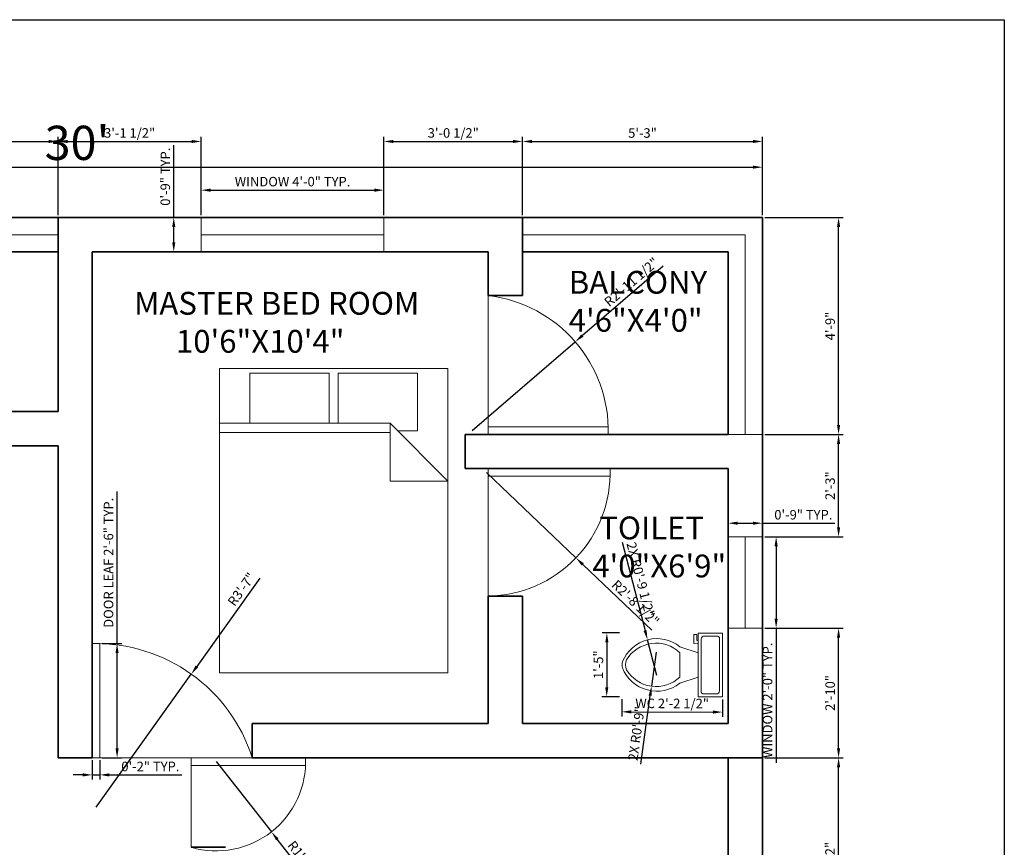
# Model space of a CAD drawing. Units: inches. Extents: x 5717 to 6221, y 11359 to 11763.
# Tile 4 of 4: x 5963 to 6221, y 11546 to 11763. Entities that reach past the tile are written whole.
import ezdxf

# ---------------------------------------------------------------- set-up
doc = ezdxf.new("R2010")
doc.units = ezdxf.units.IN
for name, color, linetype, lineweight, true_color in [('A-ANNO-DIMS', 254, 'Continuous', 13, 0xfeeab9), ('A-ANNO-TTLB', 51, 'Continuous', 25, 0xf8f6b0), ('A-AREA-IDEN', 11, 'Continuous', 20, 0xf27172), ('A-WALL', 244, 'Continuous', 35, 0x991b1e)]:
    doc.layers.add(name, color=color, linetype=linetype, lineweight=lineweight, true_color=true_color)
for name, color, linetype, lineweight in [('A-DOOR', 5, 'Continuous', 18), ('A-FLOR-FIXT', 1, 'Continuous', 18), ('A-FURN', 8, 'Continuous', 18), ('A-GLAZ', 4, 'Continuous', 18)]:
    doc.layers.add(name, color=color, linetype=linetype, lineweight=lineweight)
doc.styles.get("Standard").update_dxf_attribs({"font": 'arial.ttf'})
doc.dimstyles.new('ISO-25', dxfattribs={"dimtxt": 2.5, "dimasz": 2.5, "dimexe": 1.25, "dimexo": 0.625, "dimtad": 1, "dimlunit": 3, "dimtxsty": 'Standard', "dimcen": 2.5, "dimadec": 0, "dimazin": 0, "dimtfac": 1, "dimtmove": 0, "dimatfit": 3, "dimfxl": 1, "dimarcsym": 0})

# ---------------------------------------------------------------- blocks, each defined once
blk = doc.blocks.new('*D12')
at = {"layer": 'A-ANNO-DIMS', "color": 0, "lineweight": -2, "transparency": 16777216}
for p, q in [((5797.9, 11711.73), (5797.9, 11725.6)), ((6157.9, 11711.73), (6157.9, 11725.6)), ((5800.4, 11724.35), (6155.4, 11724.35))]:
    blk.add_line(p, q, dxfattribs=at)
at = {"layer": 'A-ANNO-DIMS', "color": 0, "transparency": 16777216}
for points in [[(5800.4, 11724.77), (5800.4, 11723.94), (5797.9, 11724.35)], [(6155.4, 11724.77), (6155.4, 11723.94), (6157.9, 11724.35)]]:
    blk.add_solid(points, dxfattribs=at)
at = {"layer": 'Defpoints', "color": 0, "transparency": 16777216}
for p in [(6157.9, 11724.35), (5797.9, 11711.11), (6157.9, 11711.11)]:
    blk.add_point(p, dxfattribs=at)
at = {"layer": 'A-ANNO-DIMS', "color": 0, "transparency": 16777216, "insert": (5977.9, 11729.58), "char_height": 9, "attachment_point": 5}
blk.add_mtext("30'", dxfattribs=at)
blk = doc.blocks.new('Toilet - top')
for p, q in [((9.5, -6), (9.5, -2)), ((-10, -8.5), (-8, -8.5)), ((-10, -9.5), (-10, -8.5)), ((-7, -9.5), (-10, -9.5)), ((-8, -8.5), (-8, -8)), ((-7, -8), (-7, -9.5)), ((-4, -8), (-6, -14)), ((4, -8), (6, -14)), ((4, -14), (-4, -14))]:
    blk.add_line(p, q)
blk.add_lwpolyline([(10.5, -8), (10.5, 0), (-10.5, 0), (-10.5, -8)], close=True)
for points in [[(-9.5, -2), (-9.5, -6)], [(8.5, -1), (-8.5, -1)], [(-8.5, -7), (8.5, -7)]]:
    blk.add_lwpolyline(points)
for centre, radius, start, end in [((-8.62, -1.88), 0.884, 81.8699, 188.1301), ((8.62, -1.88), 0.884, 351.8699, 98.1301), ((-8.62, -6.12), 0.884, 171.8699, 278.1301), ((8.62, -6.12), 0.884, 261.8699, 8.1301), ((3.52, -21.58), 12.17, 141.4691, 247.9714), ((4.2, -21.82), 11.33, 136.3677, 238.9468), ((-3.52, -21.58), 12.17, 292.0284, 38.5307), ((-4.2, -21.82), 11.33, 301.053, 43.6321), ((0, -27.88), 4, 245.7318, 294.2682), ((0, -29), 4, 254.8605, 285.1395)]:
    blk.add_arc(centre, radius, start, end)
blk = doc.blocks.new('Bed - Queen')
for p, q in [((0, -80.00003), (0, 0)), ((0, 0), (59.99999, 0)), ((59.99999, 0), (59.99999, -80.00003)), ((7.99999, -1.2), (28.79998, -1.2)), ((7.99999, -14.4), (7.99999, -1.2)), ((28.79998, -1.2), (28.79998, -14.4)), ((31.19999, -1.2), (51.99999, -1.2)), ((31.19999, -14.4), (31.19999, -1.2)), ((51.99999, -1.2), (51.99999, -16.4)), ((0, -14.4), (44.8, -14.4)), ((59.99999, -29.6), (44.8, -14.4)), ((44.8, -14.4), (44.8, -29.6)), ((44.8, -16.8), (0, -16.8)), ((51.99999, -16.4), (46.79936, -16.4)), ((44.8, -29.6), (59.99999, -29.6)), ((59.99999, -80.00003), (0, -80.00003))]:
    blk.add_line(p, q)
blk = doc.blocks.new('DOOR-LEAF-30IN')
for p, q in [((2, 30), (0, 30)), ((0, 30), (0, 0)), ((2, 0), (2, 30))]:
    blk.add_line(p, q)
blk = doc.blocks.new('WIN-24IN')
for p, q in [((0, 9), (0, 0)), ((24, 9), (0, 9)), ((24, 9), (24, 0)), ((24, 0), (24, 9)), ((0, 4.5), (24, 4.5)), ((0, 0), (24, 0))]:
    blk.add_line(p, q)
blk = doc.blocks.new('WIN-48IN')
for p, q in [((0, 0), (0, 9)), ((0, 9), (48, 9)), ((48, 9), (48, 0)), ((0, 4.5), (48, 4.5)), ((48, 0), (0, 0))]:
    blk.add_line(p, q)
blk = doc.blocks.new('*D18')
at = {"layer": 'A-ANNO-DIMS', "color": 0, "lineweight": -2, "transparency": 16777216}
for p, q in [((5988.4, 11599.11), (5988.4, 11639.13)), ((5984.53, 11599.11), (5989.65, 11599.11)), ((5988.4, 11571.61), (5988.4, 11596.61)), ((5984.53, 11569.11), (5989.65, 11569.11))]:
    blk.add_line(p, q, dxfattribs=at)
at = {"layer": 'A-ANNO-DIMS', "color": 0, "transparency": 16777216}
for points in [[(5987.99, 11596.61), (5988.82, 11596.61), (5988.4, 11599.11)], [(5987.99, 11571.61), (5988.82, 11571.61), (5988.4, 11569.11)]]:
    blk.add_solid(points, dxfattribs=at)
at = {"layer": 'Defpoints', "color": 0, "transparency": 16777216}
for p in [(5983.9, 11599.11), (5988.4, 11599.11), (5983.9, 11569.11)]:
    blk.add_point(p, dxfattribs=at)
at = {"layer": 'A-ANNO-DIMS', "color": 0, "transparency": 16777216, "insert": (5986.48, 11620.37), "char_height": 2.5, "attachment_point": 5, "rotation": 90}
blk.add_mtext('DOOR LEAF 2\'-6" TYP.', dxfattribs=at)
blk = doc.blocks.new('*D19')
at = {"layer": 'A-ANNO-DIMS', "color": 0, "lineweight": -2, "transparency": 16777216}
for p, q in [((5981.9, 11568.48), (5981.9, 11563.36)), ((5983.9, 11568.48), (5983.9, 11563.36)), ((5979.4, 11564.61), (5976.9, 11564.61)), ((5981.9, 11564.61), (5983.9, 11564.61)), ((5986.4, 11564.61), (6005.39, 11564.61))]:
    blk.add_line(p, q, dxfattribs=at)
at = {"layer": 'A-ANNO-DIMS', "color": 0, "transparency": 16777216}
for points in [[(5979.4, 11565.03), (5979.4, 11564.19), (5981.9, 11564.61)], [(5986.4, 11565.03), (5986.4, 11564.19), (5983.9, 11564.61)]]:
    blk.add_solid(points, dxfattribs=at)
at = {"layer": 'Defpoints', "color": 0, "transparency": 16777216}
for p in [(5981.9, 11569.11), (5983.9, 11569.11), (5983.9, 11564.61)]:
    blk.add_point(p, dxfattribs=at)
at = {"layer": 'A-ANNO-DIMS', "color": 0, "transparency": 16777216, "insert": (5997.15, 11566.51), "char_height": 2.5, "attachment_point": 5}
blk.add_mtext('0\'-2" TYP.', dxfattribs=at)
blk = doc.blocks.new('*D24')
at = {"layer": 'A-ANNO-DIMS', "color": 0, "lineweight": -2, "transparency": 16777216}
for p, q in [((6158.53, 11627.17), (6162.75, 11627.17)), ((6161.5, 11624.67), (6161.5, 11605.67)), ((6158.53, 11603.17), (6162.75, 11603.17)), ((6161.5, 11603.17), (6161.5, 11567.78))]:
    blk.add_line(p, q, dxfattribs=at)
at = {"layer": 'A-ANNO-DIMS', "color": 0, "transparency": 16777216}
for points in [[(6161.09, 11624.67), (6161.92, 11624.67), (6161.5, 11627.17)], [(6161.09, 11605.67), (6161.92, 11605.67), (6161.5, 11603.17)]]:
    blk.add_solid(points, dxfattribs=at)
at = {"layer": 'Defpoints', "color": 0, "transparency": 16777216}
for p in [(6157.9, 11627.17), (6157.9, 11603.17), (6161.5, 11603.17)]:
    blk.add_point(p, dxfattribs=at)
at = {"layer": 'A-ANNO-DIMS', "color": 0, "transparency": 16777216, "insert": (6159.58, 11584.22), "char_height": 2.5, "attachment_point": 5, "rotation": 90}
blk.add_mtext('WINDOW 2\'-0" TYP.', dxfattribs=at)
blk = doc.blocks.new('*D25')
at = {"layer": 'A-ANNO-DIMS', "color": 0, "lineweight": -2, "transparency": 16777216}
for p, q in [((6148.9, 11627.79), (6148.9, 11632.02)), ((6151.4, 11630.77), (6155.4, 11630.77)), ((6157.9, 11627.79), (6157.9, 11632.02)), ((6157.9, 11630.77), (6176.89, 11630.77))]:
    blk.add_line(p, q, dxfattribs=at)
at = {"layer": 'A-ANNO-DIMS', "color": 0, "transparency": 16777216}
for points in [[(6151.4, 11631.18), (6151.4, 11630.35), (6148.9, 11630.77)], [(6155.4, 11631.18), (6155.4, 11630.35), (6157.9, 11630.77)]]:
    blk.add_solid(points, dxfattribs=at)
at = {"layer": 'Defpoints', "color": 0, "transparency": 16777216}
for p in [(6157.9, 11630.77), (6148.9, 11627.17), (6157.9, 11627.17)]:
    blk.add_point(p, dxfattribs=at)
at = {"layer": 'A-ANNO-DIMS', "color": 0, "transparency": 16777216, "insert": (6168.65, 11632.67), "char_height": 2.5, "attachment_point": 5}
blk.add_mtext('0\'-9" TYP.', dxfattribs=at)
blk = doc.blocks.new('*D26')
at = {"layer": 'A-ANNO-DIMS', "color": 0, "lineweight": -2, "transparency": 16777216}
for p, q in [((6010.49, 11711.73), (6010.49, 11719.56)), ((6012.99, 11718.31), (6055.99, 11718.31)), ((6058.49, 11711.73), (6058.49, 11719.56))]:
    blk.add_line(p, q, dxfattribs=at)
at = {"layer": 'A-ANNO-DIMS', "color": 0, "transparency": 16777216}
for points in [[(6012.99, 11718.73), (6012.99, 11717.89), (6010.49, 11718.31)], [(6055.99, 11718.73), (6055.99, 11717.89), (6058.49, 11718.31)]]:
    blk.add_solid(points, dxfattribs=at)
at = {"layer": 'Defpoints', "color": 0, "transparency": 16777216}
for p in [(6058.49, 11718.31), (6010.49, 11711.11), (6058.49, 11711.11)]:
    blk.add_point(p, dxfattribs=at)
at = {"layer": 'A-ANNO-DIMS', "color": 0, "transparency": 16777216, "insert": (6034.49, 11720.23), "char_height": 2.5, "attachment_point": 5}
blk.add_mtext('WINDOW 4\'-0" TYP.', dxfattribs=at)
blk = doc.blocks.new('*D27')
at = {"layer": 'A-ANNO-DIMS', "color": 0, "lineweight": -2, "transparency": 16777216}
for p, q in [((6003.29, 11711.11), (6003.29, 11730.1)), ((6009.87, 11711.11), (6002.04, 11711.11)), ((6003.29, 11704.61), (6003.29, 11708.61)), ((6009.87, 11702.11), (6002.04, 11702.11))]:
    blk.add_line(p, q, dxfattribs=at)
at = {"layer": 'A-ANNO-DIMS', "color": 0, "transparency": 16777216}
for points in [[(6002.87, 11708.61), (6003.71, 11708.61), (6003.29, 11711.11)], [(6002.87, 11704.61), (6003.71, 11704.61), (6003.29, 11702.11)]]:
    blk.add_solid(points, dxfattribs=at)
at = {"layer": 'Defpoints', "color": 0, "transparency": 16777216}
for p in [(6003.29, 11711.11), (6010.49, 11711.11), (6010.49, 11702.11)]:
    blk.add_point(p, dxfattribs=at)
at = {"layer": 'A-ANNO-DIMS', "color": 0, "transparency": 16777216, "insert": (6001.39, 11721.85), "char_height": 2.5, "attachment_point": 5, "rotation": 90}
blk.add_mtext('0\'-9" TYP.', dxfattribs=at)
blk = doc.blocks.new('*D30')
at = {"layer": 'A-ANNO-DIMS', "color": 0, "lineweight": -2, "transparency": 16777216}
for p, q in [((6120.97, 11584.53), (6120.96, 11579.94)), ((6147.41, 11584.46), (6147.4, 11579.87)), ((6123.46, 11581.18), (6144.9, 11581.13))]:
    blk.add_line(p, q, dxfattribs=at)
at = {"layer": 'A-ANNO-DIMS', "color": 0, "transparency": 16777216}
for points in [[(6123.46, 11581.6), (6123.46, 11580.77), (6120.96, 11581.19)], [(6144.9, 11581.55), (6144.9, 11580.71), (6147.4, 11581.12)]]:
    blk.add_solid(points, dxfattribs=at)
at = {"layer": 'Defpoints', "color": 0, "transparency": 16777216}
for p in [(6120.97, 11585.15), (6147.41, 11585.09), (6147.4, 11581.12)]:
    blk.add_point(p, dxfattribs=at)
at = {"layer": 'A-ANNO-DIMS', "color": 0, "transparency": 16777216, "insert": (6134.19, 11583.07), "char_height": 2.5, "attachment_point": 5, "rotation": 359.8573}
blk.add_mtext('WC 2\'-2 1/2"', dxfattribs=at)
blk = doc.blocks.new('*D31')
at = {"layer": 'A-ANNO-DIMS', "color": 0, "lineweight": -2, "transparency": 16777216}
for p, q in [((6120.39, 11601.96), (6115.8, 11601.97)), ((6117.04, 11599.46), (6117.01, 11587.66)), ((6120.35, 11585.16), (6115.76, 11585.17))]:
    blk.add_line(p, q, dxfattribs=at)
at = {"layer": 'A-ANNO-DIMS', "color": 0, "transparency": 16777216}
for points in [[(6116.63, 11599.47), (6117.46, 11599.46), (6117.05, 11601.96)], [(6116.6, 11587.67), (6117.43, 11587.66), (6117.01, 11585.16)]]:
    blk.add_solid(points, dxfattribs=at)
at = {"layer": 'Defpoints', "color": 0, "transparency": 16777216}
for p in [(6121.02, 11601.95), (6117.01, 11585.16), (6120.97, 11585.15)]:
    blk.add_point(p, dxfattribs=at)
at = {"layer": 'A-ANNO-DIMS', "color": 0, "transparency": 16777216, "insert": (6115.13, 11593.57), "char_height": 2.5, "attachment_point": 5, "rotation": 89.8573}
blk.add_mtext('1\'-5"', dxfattribs=at)
blk = doc.blocks.new('*D43')
at = {"layer": 'A-ANNO-DIMS', "color": 0, "lineweight": -2, "transparency": 16777216}
for p, q in [((6158.53, 11569.11), (6179.15, 11569.11)), ((6177.9, 11513.97), (6177.9, 11566.61)), ((6158.53, 11511.47), (6179.15, 11511.47))]:
    blk.add_line(p, q, dxfattribs=at)
at = {"layer": 'A-ANNO-DIMS', "color": 0, "transparency": 16777216}
for points in [[(6177.49, 11566.61), (6178.32, 11566.61), (6177.9, 11569.11)], [(6177.49, 11513.97), (6178.32, 11513.97), (6177.9, 11511.47)]]:
    blk.add_solid(points, dxfattribs=at)
at = {"layer": 'Defpoints', "color": 0, "transparency": 16777216}
for p in [(6157.9, 11569.11), (6177.9, 11569.11), (6157.9, 11511.47)]:
    blk.add_point(p, dxfattribs=at)
at = {"layer": 'A-ANNO-DIMS', "color": 0, "transparency": 16777216, "insert": (6175.98, 11540.29), "char_height": 2.5, "attachment_point": 5, "rotation": 90}
blk.add_mtext('4\'-9 1/2"', dxfattribs=at)
blk = doc.blocks.new('*D44')
at = {"layer": 'A-ANNO-DIMS', "color": 0, "lineweight": -2, "transparency": 16777216}
for p, q in [((6158.53, 11603.17), (6179.15, 11603.17)), ((6177.9, 11571.61), (6177.9, 11600.67)), ((6158.53, 11569.11), (6179.15, 11569.11))]:
    blk.add_line(p, q, dxfattribs=at)
at = {"layer": 'A-ANNO-DIMS', "color": 0, "transparency": 16777216}
for points in [[(6177.49, 11600.67), (6178.32, 11600.67), (6177.9, 11603.17)], [(6177.49, 11571.61), (6178.32, 11571.61), (6177.9, 11569.11)]]:
    blk.add_solid(points, dxfattribs=at)
at = {"layer": 'Defpoints', "color": 0, "transparency": 16777216}
for p in [(6157.9, 11603.17), (6177.9, 11603.17), (6157.9, 11569.11)]:
    blk.add_point(p, dxfattribs=at)
at = {"layer": 'A-ANNO-DIMS', "color": 0, "transparency": 16777216, "insert": (6176, 11586.14), "char_height": 2.5, "attachment_point": 5, "rotation": 90}
blk.add_mtext('2\'-10"', dxfattribs=at)
blk = doc.blocks.new('*D45')
at = {"layer": 'A-ANNO-DIMS', "color": 0, "lineweight": -2, "transparency": 16777216}
for p, q in [((6158.53, 11654.11), (6179.15, 11654.11)), ((6177.9, 11629.67), (6177.9, 11651.61)), ((6158.53, 11627.17), (6179.15, 11627.17))]:
    blk.add_line(p, q, dxfattribs=at)
at = {"layer": 'A-ANNO-DIMS', "color": 0, "transparency": 16777216}
for points in [[(6177.49, 11651.61), (6178.32, 11651.61), (6177.9, 11654.11)], [(6177.49, 11629.67), (6178.32, 11629.67), (6177.9, 11627.17)]]:
    blk.add_solid(points, dxfattribs=at)
at = {"layer": 'Defpoints', "color": 0, "transparency": 16777216}
for p in [(6157.9, 11654.11), (6177.9, 11654.11), (6157.9, 11627.17)]:
    blk.add_point(p, dxfattribs=at)
at = {"layer": 'A-ANNO-DIMS', "color": 0, "transparency": 16777216, "insert": (6176, 11640.64), "char_height": 2.5, "attachment_point": 5, "rotation": 90}
blk.add_mtext('2\'-3"', dxfattribs=at)
blk = doc.blocks.new('*D46')
at = {"layer": 'A-ANNO-DIMS', "color": 0, "lineweight": -2, "transparency": 16777216}
for p, q in [((6158.53, 11711.11), (6179.15, 11711.11)), ((6177.9, 11656.61), (6177.9, 11708.61)), ((6158.53, 11654.11), (6179.15, 11654.11))]:
    blk.add_line(p, q, dxfattribs=at)
at = {"layer": 'A-ANNO-DIMS', "color": 0, "transparency": 16777216}
for points in [[(6177.49, 11708.61), (6178.32, 11708.61), (6177.9, 11711.11)], [(6177.49, 11656.61), (6178.32, 11656.61), (6177.9, 11654.11)]]:
    blk.add_solid(points, dxfattribs=at)
at = {"layer": 'Defpoints', "color": 0, "transparency": 16777216}
for p in [(6157.9, 11711.11), (6177.9, 11711.11), (6157.9, 11654.11)]:
    blk.add_point(p, dxfattribs=at)
at = {"layer": 'A-ANNO-DIMS', "color": 0, "transparency": 16777216, "insert": (6176, 11682.61), "char_height": 2.5, "attachment_point": 5, "rotation": 90}
blk.add_mtext('4\'-9"', dxfattribs=at)
blk = doc.blocks.new('*D51')
at = {"layer": 'A-ANNO-DIMS', "color": 0, "lineweight": -2, "transparency": 16777216}
for p, q in [((5886.11, 11711.73), (5886.11, 11732.36)), ((5888.61, 11731.11), (5970.4, 11731.11)), ((5972.9, 11711.73), (5972.9, 11732.36))]:
    blk.add_line(p, q, dxfattribs=at)
at = {"layer": 'A-ANNO-DIMS', "color": 0, "transparency": 16777216}
for points in [[(5888.61, 11731.53), (5888.61, 11730.69), (5886.11, 11731.11)], [(5970.4, 11731.53), (5970.4, 11730.69), (5972.9, 11731.11)]]:
    blk.add_solid(points, dxfattribs=at)
at = {"layer": 'Defpoints', "color": 0, "transparency": 16777216}
for p in [(5972.9, 11731.11), (5886.11, 11711.11), (5972.9, 11711.11)]:
    blk.add_point(p, dxfattribs=at)
at = {"layer": 'A-ANNO-DIMS', "color": 0, "transparency": 16777216, "insert": (5929.51, 11733.01), "char_height": 2.5, "attachment_point": 5}
blk.add_mtext('7\'-3"', dxfattribs=at)
blk = doc.blocks.new('*D52')
at = {"layer": 'A-ANNO-DIMS', "color": 0, "lineweight": -2, "transparency": 16777216}
for p, q in [((5972.9, 11711.73), (5972.9, 11732.36)), ((5975.4, 11731.11), (6007.99, 11731.11)), ((6010.49, 11711.73), (6010.49, 11732.36))]:
    blk.add_line(p, q, dxfattribs=at)
at = {"layer": 'A-ANNO-DIMS', "color": 0, "transparency": 16777216}
for points in [[(5975.4, 11731.53), (5975.4, 11730.69), (5972.9, 11731.11)], [(6007.99, 11731.53), (6007.99, 11730.69), (6010.49, 11731.11)]]:
    blk.add_solid(points, dxfattribs=at)
at = {"layer": 'Defpoints', "color": 0, "transparency": 16777216}
for p in [(6010.49, 11731.11), (5972.9, 11711.11), (6010.49, 11711.11)]:
    blk.add_point(p, dxfattribs=at)
at = {"layer": 'A-ANNO-DIMS', "color": 0, "transparency": 16777216, "insert": (5991.7, 11733.03), "char_height": 2.5, "attachment_point": 5}
blk.add_mtext('3\'-1 1/2"', dxfattribs=at)
blk = doc.blocks.new('*D53')
at = {"layer": 'A-ANNO-DIMS', "color": 0, "lineweight": -2, "transparency": 16777216}
for p, q in [((6058.49, 11711.73), (6058.49, 11732.36)), ((6060.99, 11731.11), (6092.4, 11731.11)), ((6094.9, 11711.73), (6094.9, 11732.36))]:
    blk.add_line(p, q, dxfattribs=at)
at = {"layer": 'A-ANNO-DIMS', "color": 0, "transparency": 16777216}
for points in [[(6060.99, 11731.53), (6060.99, 11730.69), (6058.49, 11731.11)], [(6092.4, 11731.53), (6092.4, 11730.69), (6094.9, 11731.11)]]:
    blk.add_solid(points, dxfattribs=at)
at = {"layer": 'Defpoints', "color": 0, "transparency": 16777216}
for p in [(6094.9, 11731.11), (6058.49, 11711.11), (6094.9, 11711.11)]:
    blk.add_point(p, dxfattribs=at)
at = {"layer": 'A-ANNO-DIMS', "color": 0, "transparency": 16777216, "insert": (6076.7, 11733.03), "char_height": 2.5, "attachment_point": 5}
blk.add_mtext('3\'-0 1/2"', dxfattribs=at)
blk = doc.blocks.new('*D54')
at = {"layer": 'A-ANNO-DIMS', "color": 0, "lineweight": -2, "transparency": 16777216}
for p, q in [((6094.9, 11711.73), (6094.9, 11732.36)), ((6097.4, 11731.11), (6155.4, 11731.11)), ((6157.9, 11711.73), (6157.9, 11732.36))]:
    blk.add_line(p, q, dxfattribs=at)
at = {"layer": 'A-ANNO-DIMS', "color": 0, "transparency": 16777216}
for points in [[(6097.4, 11731.53), (6097.4, 11730.69), (6094.9, 11731.11)], [(6155.4, 11731.53), (6155.4, 11730.69), (6157.9, 11731.11)]]:
    blk.add_solid(points, dxfattribs=at)
at = {"layer": 'Defpoints', "color": 0, "transparency": 16777216}
for p in [(6157.9, 11731.11), (6094.9, 11711.11), (6157.9, 11711.11)]:
    blk.add_point(p, dxfattribs=at)
at = {"layer": 'A-ANNO-DIMS', "color": 0, "transparency": 16777216, "insert": (6126.4, 11733.01), "char_height": 2.5, "attachment_point": 5}
blk.add_mtext('5\'-3"', dxfattribs=at)
blk = doc.blocks.new('*D60')
at = {"layer": 'A-ANNO-DIMS', "color": 0, "lineweight": -2, "transparency": 16777216}
for p, q in [((6025.89, 11616.3), (6009.36, 11593.14)), ((5982.9, 11556.11), (6007.9, 11591.11))]:
    blk.add_line(p, q, dxfattribs=at)
at = {"layer": 'A-ANNO-DIMS', "color": 0, "transparency": 16777216}
blk.add_solid([(6009.02, 11593.39), (6009.69, 11592.9), (6007.9, 11591.11)], dxfattribs=at)
at = {"layer": 'Defpoints', "color": 0, "transparency": 16777216}
for p in [(6007.9, 11591.11), (5982.9, 11556.11)]:
    blk.add_point(p, dxfattribs=at)
at = {"layer": 'A-ANNO-DIMS', "color": 0, "transparency": 16777216, "insert": (6021.35, 11613.21), "char_height": 2.5, "attachment_point": 5, "rotation": 54.4628}
blk.add_mtext('R3\'-7"', dxfattribs=at)
blk = doc.blocks.new('*D61')
at = {"layer": 'A-ANNO-DIMS', "color": 0, "lineweight": -2, "transparency": 16777216}
for p, q in [((6131.79, 11698.37), (6110.62, 11680.09)), ((6081.69, 11655.11), (6108.73, 11678.46))]:
    blk.add_line(p, q, dxfattribs=at)
at = {"layer": 'A-ANNO-DIMS', "color": 0, "transparency": 16777216}
blk.add_solid([(6110.35, 11680.41), (6110.89, 11679.78), (6108.73, 11678.46)], dxfattribs=at)
at = {"layer": 'Defpoints', "color": 0, "transparency": 16777216}
for p in [(6108.73, 11678.46), (6081.69, 11655.11)]:
    blk.add_point(p, dxfattribs=at)
at = {"layer": 'A-ANNO-DIMS', "color": 0, "transparency": 16777216, "insert": (6123.7, 11693.92), "char_height": 2.5, "attachment_point": 5, "rotation": 40.8133}
blk.add_mtext('R2\'-11 1/2"', dxfattribs=at)
blk = doc.blocks.new('*D62')
at = {"layer": 'A-ANNO-DIMS', "color": 0, "lineweight": -2, "transparency": 16777216}
for p, q in [((6085.41, 11644.11), (6108.92, 11621.66)), ((6128.85, 11602.62), (6110.73, 11619.93))]:
    blk.add_line(p, q, dxfattribs=at)
at = {"layer": 'A-ANNO-DIMS', "color": 0, "transparency": 16777216}
blk.add_solid([(6111.01, 11620.23), (6110.44, 11619.63), (6108.92, 11621.66)], dxfattribs=at)
at = {"layer": 'Defpoints', "color": 0, "transparency": 16777216}
for p in [(6085.41, 11644.11), (6108.92, 11621.66)]:
    blk.add_point(p, dxfattribs=at)
at = {"layer": 'A-ANNO-DIMS', "color": 0, "transparency": 16777216, "insert": (6124.35, 11609.57), "char_height": 2.5, "attachment_point": 5, "rotation": 316.3127}
blk.add_mtext('R2\'-8 1/2"', dxfattribs=at)
blk = doc.blocks.new('*D66')
at = {"layer": 'A-ANNO-DIMS', "color": 0, "lineweight": -2, "transparency": 16777216}
for p, q in [((6014.46, 11568.11), (6028.94, 11549.64)), ((6043.2, 11531.46), (6030.48, 11547.68))]:
    blk.add_line(p, q, dxfattribs=at)
at = {"layer": 'A-ANNO-DIMS', "color": 0, "transparency": 16777216}
blk.add_solid([(6030.81, 11547.93), (6030.16, 11547.42), (6028.94, 11549.64)], dxfattribs=at)
at = {"layer": 'Defpoints', "color": 0, "transparency": 16777216}
for p in [(6014.46, 11568.11), (6028.94, 11549.64)]:
    blk.add_point(p, dxfattribs=at)
at = {"layer": 'A-ANNO-DIMS', "color": 0, "transparency": 16777216, "insert": (6039.14, 11539.75), "char_height": 2.5, "attachment_point": 5, "rotation": 308.1145}
blk.add_mtext('R1\'-11 1/2"', dxfattribs=at)
blk = doc.blocks.new('*D70')
at = {"layer": 'A-ANNO-DIMS', "color": 0, "lineweight": -2, "transparency": 16777216}
for p, q in [((6121.03, 11625.81), (6127.08, 11602.56)), ((6130.16, 11590.72), (6127.71, 11600.14))]:
    blk.add_line(p, q, dxfattribs=at)
at = {"layer": 'A-ANNO-DIMS', "color": 0, "transparency": 16777216}
blk.add_solid([(6127.48, 11602.66), (6126.68, 11602.45), (6127.71, 11600.14)], dxfattribs=at)
at = {"layer": 'Defpoints', "color": 0, "transparency": 16777216}
for p in [(6127.71, 11600.14), (6130.16, 11590.72)]:
    blk.add_point(p, dxfattribs=at)
at = {"layer": 'A-ANNO-DIMS', "color": 0, "transparency": 16777216, "insert": (6125.6, 11615.88), "char_height": 2.5, "attachment_point": 5, "rotation": 284.575}
blk.add_mtext('2X R0\'-9 1/2"', dxfattribs=at)
blk = doc.blocks.new('*D71')
at = {"layer": 'A-ANNO-DIMS', "color": 0, "lineweight": -2, "transparency": 16777216}
for p, q in [((6129.99, 11596.89), (6128.76, 11587.91)), ((6125.95, 11567.4), (6128.42, 11585.44))]:
    blk.add_line(p, q, dxfattribs=at)
at = {"layer": 'A-ANNO-DIMS', "color": 0, "transparency": 16777216}
blk.add_solid([(6128, 11585.49), (6128.83, 11585.38), (6128.76, 11587.91)], dxfattribs=at)
at = {"layer": 'Defpoints', "color": 0, "transparency": 16777216}
for p in [(6129.99, 11596.89), (6128.76, 11587.91)]:
    blk.add_point(p, dxfattribs=at)
at = {"layer": 'A-ANNO-DIMS', "color": 0, "transparency": 16777216, "insert": (6125.13, 11575.44), "char_height": 2.5, "attachment_point": 5, "rotation": 82.2016}
blk.add_mtext('2X R0\'-9"', dxfattribs=at)

msp = doc.modelspace()

# ---------------------------------------------------------------- linework, layer by layer
at = {"layer": 'A-ANNO-TTLB'}
msp.add_lwpolyline([(5717.423, 11763.126), (6221.432, 11763.126), (6221.432, 11381.867), (5717.423, 11381.867)], close=True, dxfattribs=at)
at = {"layer": 'A-DOOR'}
for p, q in [((6085.902, 11654.109), (6085.902, 11690.584)), ((6085.902, 11656.109), (6117.402, 11656.109)), ((6117.402, 11654.109), (6117.402, 11656.109)), ((6085.902, 11654.109), (6117.402, 11654.109)), ((6085.902, 11611.609), (6085.902, 11645.109)), ((6085.902, 11645.109), (6115.902, 11645.109)), ((6115.902, 11645.109), (6117.902, 11645.109)), ((6117.902, 11645.109), (6117.902, 11643.109)), ((6117.902, 11643.109), (6085.902, 11643.109)), ((6023.902, 11569.109), (5981.902, 11569.109)), ((6007.902, 11569.109), (6007.902, 11545.574)), ((6007.902, 11545.574), (6007.902, 11569.109))]:
    msp.add_line(p, q, dxfattribs=at)
for centre, radius, start, end in [((6081.692, 11655.109), 35.724, 358.39594, 83.23221), ((6085.414, 11644.109), 32.504, 270.86075, 1.76303), ((5982.902, 11556.109), 43.012, 17.59242, 91.33222), ((6014.455, 11568.109), 23.469, 253.78655, 2.44213)]:
    msp.add_arc(centre, radius, start, end, dxfattribs=at)
at = {"layer": 'A-GLAZ'}
for p, q in [((5886.109, 11711.109), (5972.902, 11711.109)), ((5972.902, 11711.109), (5972.902, 11702.109)), ((6058.491, 11711.109), (6058.491, 11702.109)), ((6094.902, 11711.109), (6094.902, 11702.109)), ((6157.902, 11711.109), (6094.902, 11711.109)), ((6157.902, 11654.109), (6157.902, 11711.109)), ((5886.109, 11706.609), (5972.902, 11706.609)), ((6094.902, 11706.609), (6153.402, 11706.609)), ((6153.402, 11706.609), (6153.402, 11654.109)), ((5972.902, 11702.109), (5886.109, 11702.109)), ((6094.902, 11702.109), (6148.902, 11702.109)), ((6148.902, 11702.109), (6148.902, 11654.109)), ((6148.902, 11654.109), (6157.902, 11654.109))]:
    msp.add_line(p, q, dxfattribs=at)
at = {"layer": 'A-WALL'}
for p, q in [((6157.902, 11711.109), (5797.902, 11711.109)), ((5972.902, 11711.109), (5972.902, 11660.109)), ((6094.902, 11690.584), (6094.902, 11711.109)), ((6157.902, 11411.109), (6157.902, 11711.109)), ((5972.902, 11702.109), (5873.902, 11702.109)), ((5981.902, 11702.109), (5981.902, 11569.109)), ((6085.902, 11702.109), (5981.902, 11702.109)), ((6085.902, 11690.584), (6085.902, 11702.109)), ((6148.902, 11702.109), (6094.902, 11702.109)), ((6148.902, 11654.109), (6148.902, 11702.109)), ((6094.902, 11690.584), (6085.902, 11690.584)), ((5972.902, 11660.109), (5905.38, 11660.109)), ((6085.902, 11654.109), (6079.855, 11654.109)), ((6079.855, 11654.109), (6079.855, 11645.109)), ((6148.902, 11654.109), (6085.902, 11654.109)), ((5972.902, 11651.109), (5893.38, 11651.109)), ((5972.902, 11651.109), (5972.902, 11569.109)), ((6079.855, 11645.109), (6085.902, 11645.109)), ((6148.902, 11645.109), (6085.902, 11645.109)), ((6148.902, 11578.109), (6148.902, 11645.109)), ((6085.902, 11578.109), (6085.902, 11611.609)), ((6085.902, 11611.609), (6094.902, 11611.609)), ((6094.902, 11578.109), (6094.902, 11611.609)), ((6023.902, 11578.109), (6023.902, 11569.109)), ((6085.902, 11578.109), (6023.902, 11578.109)), ((6148.902, 11578.109), (6094.902, 11578.109)), ((5981.902, 11569.109), (5972.902, 11569.109)), ((6157.902, 11569.109), (6023.902, 11569.109)), ((6148.902, 11420.109), (6148.902, 11569.109)), ((6007.902, 11545.574), (6016.902, 11545.574))]:
    msp.add_line(p, q, dxfattribs=at)

# ---------------------------------------------------------------- block references
at = {"layer": 'A-DOOR'}
msp.add_blockref('DOOR-LEAF-30IN', (5981.902, 11569.109), dxfattribs=at)
at = {"layer": 'A-DOOR', "rotation": 269.9999999999973}
msp.add_blockref('DOOR-LEAF-30IN', (6007.902, 11569.109), dxfattribs=at)
at = {"layer": 'A-FLOR-FIXT', "xscale": 0.8, "yscale": 0.8, "zscale": 0.8, "rotation": 269.8573235380506}
msp.add_blockref('Toilet - top', (6147.431, 11593.489), dxfattribs=at)
at = {"layer": 'A-FURN'}
msp.add_blockref('Bed - Queen', (6015.302, 11671.446), dxfattribs=at)
at = {"layer": 'A-GLAZ'}
msp.add_blockref('WIN-48IN', (6010.491, 11702.109), dxfattribs=at)
at = {"layer": 'A-GLAZ', "rotation": 270.0000000000009}
msp.add_blockref('WIN-24IN', (6148.902, 11627.167), dxfattribs=at)

# ---------------------------------------------------------------- texts
at = {"layer": 'A-AREA-IDEN', "char_height": 6, "attachment_point": 1}
for s, insert in [('  BALCONY\\P  4\'6"X4\'0"', (6103.364, 11697.098)), ('MASTER BED ROOM\\P      10\'6"X10\'4"', (5992.872, 11691.577)), (' TOILET\\P4\'0"X6\'9"', (6113.214, 11632.529))]:
    msp.add_mtext_dynamic_manual_height_columns(s, width=116.60264, gutter_width=12.5, heights=[0], dxfattribs=dict(at, insert=insert))

# ---------------------------------------------------------------- dimensions: what is measured, and where the dimension line sits
at = {"layer": 'A-ANNO-DIMS'}
for base, p1, p2, override, picture, middle in [((6157.902, 11724.352), (5797.902, 11711.109), (6157.902, 11711.109), {"dimtxt": 9, "dimclrd": 0, "dimclre": 0, "dimclrt": 0}, '*D12', (5977.902, 11729.575)), ((6010.491, 11731.109), (5972.902, 11711.109), (6010.491, 11711.109), {"dimdec": 1, "dimlfac": 1, "dimrnd": 0, "dimzin": 1, "dimdsep": 46, "dimlunit": 4, "dimfrac": 2}, '*D52', (5991.697, 11733.027)), ((5972.902, 11731.109), (5886.109, 11711.109), (5972.902, 11711.109), {"dimdec": 1, "dimlfac": 1, "dimrnd": 0, "dimzin": 1, "dimdsep": 46, "dimlunit": 4, "dimfrac": 2}, '*D51', (5929.506, 11733.011)), ((6157.902, 11731.109), (6094.902, 11711.109), (6157.902, 11711.109), {"dimdec": 1, "dimlfac": 1, "dimrnd": 0, "dimzin": 1, "dimdsep": 46, "dimlunit": 4, "dimfrac": 2}, '*D54', (6126.402, 11733.011))]:
    dim = msp.add_linear_dim(base=base, p1=p1, p2=p2, dimstyle='ISO-25', override=override, dxfattribs=at)
    dim.commit()
    dim.dimension.update_dxf_attribs({"geometry": picture, "text_midpoint": middle})
for base, p1, p2, angle, picture, middle in [((6094.902, 11731.109), (6058.491, 11711.109), (6094.902, 11711.109), 0, '*D53', (6076.697, 11733.027)), ((6177.902, 11711.109), (6157.902, 11654.109), (6157.902, 11711.109), 90, '*D46', (6176.001, 11682.609)), ((6177.902, 11654.109), (6157.902, 11627.167), (6157.902, 11654.109), 90, '*D45', (6176, 11640.638)), ((6117.008, 11585.164), (6121.015, 11601.955), (6120.973, 11585.155), 269.85732, '*D31', (6115.127, 11593.569)), ((6177.902, 11603.167), (6157.902, 11569.109), (6157.902, 11603.167), 90, '*D44', (6176.001, 11586.138)), ((6177.902, 11569.109), (6157.902, 11511.47), (6157.902, 11569.109), 90, '*D43', (6175.985, 11540.29))]:
    dim = msp.add_linear_dim(base=base, p1=p1, p2=p2, angle=angle, dimstyle='ISO-25', override={"dimdec": 1, "dimlfac": 1, "dimrnd": 0, "dimzin": 1, "dimdsep": 46, "dimlunit": 4, "dimfrac": 2}, dxfattribs=at)
    dim.commit()
    dim.dimension.update_dxf_attribs({"geometry": picture, "text_midpoint": middle})
for base, p1, p2, angle, text, picture, middle in [((6003.291, 11711.109), (6010.491, 11702.109), (6010.491, 11711.109), 90, '<> TYP.', '*D27', (6001.39, 11721.853)), ((5988.402, 11599.109), (5983.902, 11569.109), (5983.902, 11599.109), 90, 'DOOR LEAF <> TYP.', '*D18', (5986.484, 11620.367)), ((6161.502, 11603.167), (6157.902, 11627.167), (6157.902, 11603.167), 270, 'WINDOW <> TYP.', '*D24', (6159.584, 11584.225)), ((6147.4, 11581.123), (6120.973, 11585.155), (6147.41, 11585.089), 359.85732, 'WC <>', '*D30', (6134.187, 11583.074))]:
    dim = msp.add_linear_dim(base=base, p1=p1, p2=p2, angle=angle, text=text, dimstyle='ISO-25', override={"dimdec": 1, "dimlfac": 1, "dimrnd": 0, "dimzin": 1, "dimdsep": 46, "dimlunit": 4, "dimfrac": 2}, dxfattribs=at)
    dim.commit()
    dim.dimension.update_dxf_attribs({"geometry": picture, "text_midpoint": middle})
for base, p1, p2, text, picture, middle in [((6058.491, 11718.309), (6010.491, 11711.109), (6058.491, 11711.109), 'WINDOW <> TYP.', '*D26', (6034.491, 11720.227)), ((6157.902, 11630.767), (6148.902, 11627.167), (6157.902, 11627.167), '<> TYP.', '*D25', (6168.647, 11632.669)), ((5983.902, 11564.609), (5981.902, 11569.109), (5983.902, 11569.109), '<> TYP.', '*D19', (5997.147, 11566.51))]:
    dim = msp.add_linear_dim(base=base, p1=p1, p2=p2, text=text, dimstyle='ISO-25', override={"dimdec": 1, "dimlfac": 1, "dimrnd": 0, "dimzin": 1, "dimdsep": 46, "dimlunit": 4, "dimfrac": 2}, dxfattribs=at)
    dim.commit()
    dim.dimension.update_dxf_attribs({"geometry": picture, "text_midpoint": middle})
for center, mpoint, picture, middle in [((6081.692, 11655.109), (6108.73, 11678.458), '*D61', (6124.952, 11692.467)), ((6085.414, 11644.109), (6108.918, 11621.658), '*D62', (6123.021, 11608.187)), ((5982.902, 11556.109), (6007.902, 11591.109), '*D60', (6022.902, 11612.109)), ((6014.455, 11568.109), (6028.941, 11549.644), '*D66', (6037.632, 11538.566))]:
    dim = msp.add_radius_dim(center=center, mpoint=mpoint, dimstyle='ISO-25', override={"dimdec": 1, "dimlfac": 1, "dimrnd": 0, "dimzin": 1, "dimdsep": 46, "dimlunit": 4, "dimfrac": 2}, dxfattribs=at)
    dim.commit()
    dim.dimension.update_dxf_attribs({"geometry": picture, "text_midpoint": middle, "dimtype": 164})
for center, mpoint, picture, middle in [((6130.16, 11590.716), (6127.71, 11600.138), '*D70', (6125.599, 11615.877)), ((6129.986, 11596.892), (6128.756, 11587.913), '*D71', (6125.128, 11575.438))]:
    dim = msp.add_radius_dim(center=center, mpoint=mpoint, text='2X <>', dimstyle='ISO-25', override={"dimdec": 1, "dimlfac": 1, "dimrnd": 0, "dimzin": 1, "dimdsep": 46, "dimlunit": 4, "dimfrac": 2}, dxfattribs=at)
    dim.commit()
    dim.dimension.update_dxf_attribs({"geometry": picture, "text_midpoint": middle})

doc.saveas('drawing.dxf')
